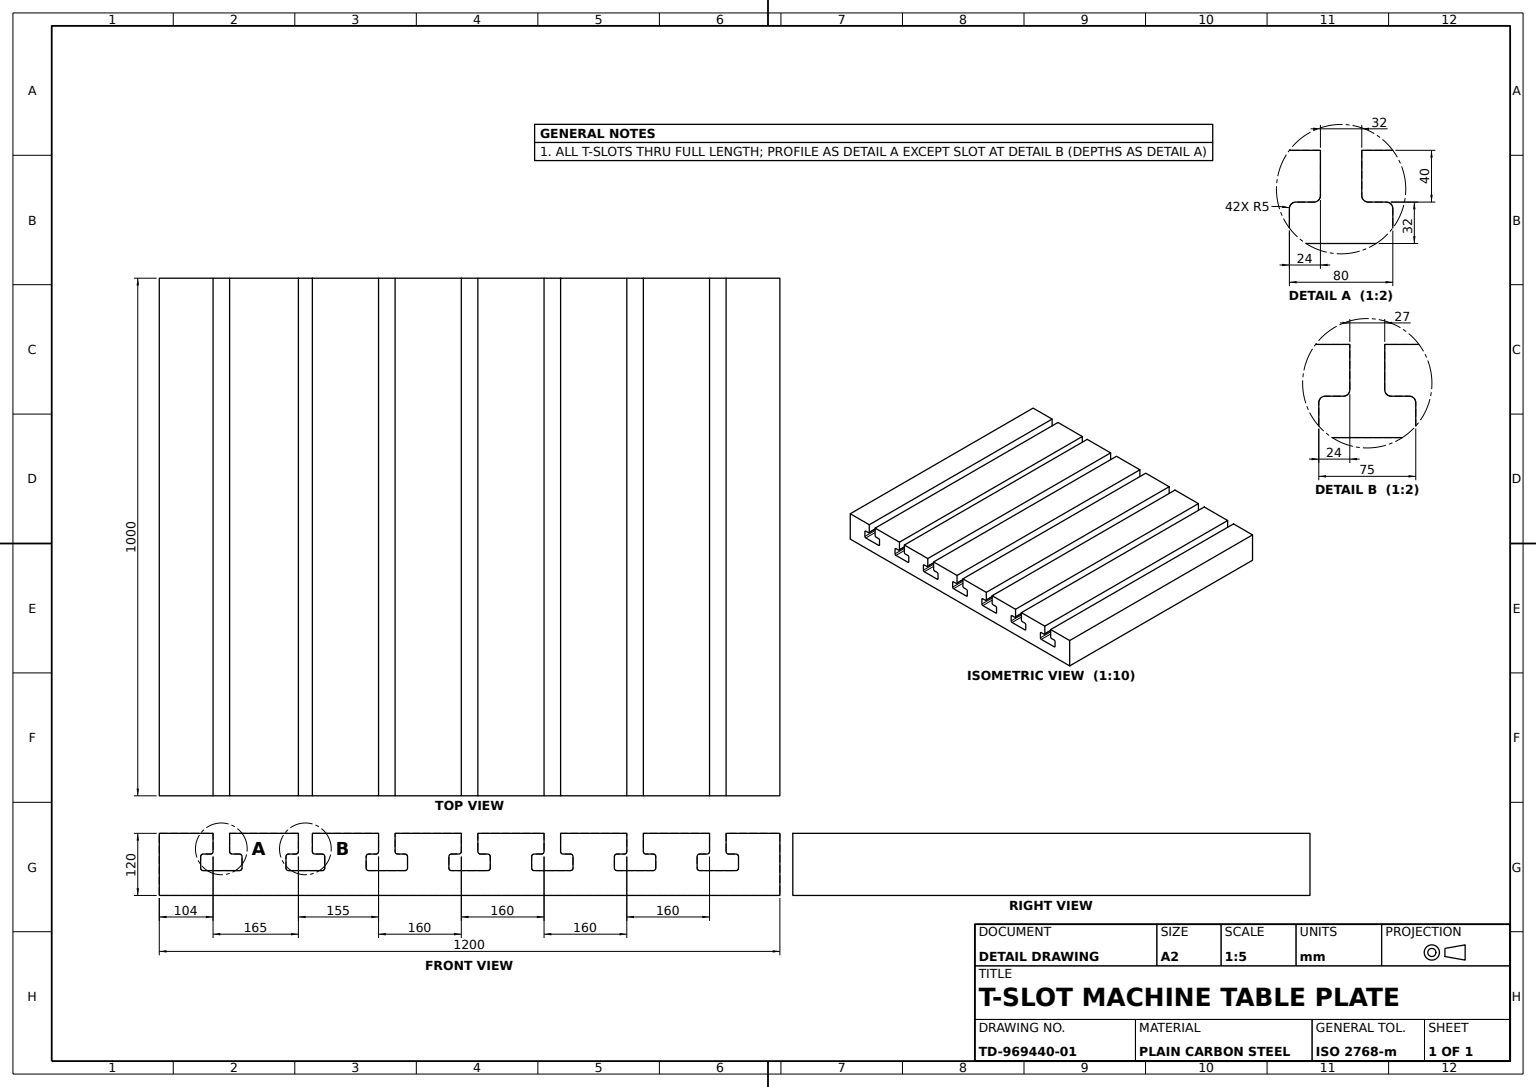
from build123d import *

# Parameters (mm, degrees)
PLATE_OUTLINE_SKETCH_W = 1200
PLATE_OUTLINE_SKETCH_H = 1000
BASE_PLATE_120MM_DEPTH = 120
T_SLOTS_SET_A_DEPTH    = 1000
T_SLOTS_SET_B_DEPTH    = 1000


with BuildPart() as part:
    # Plate Outline Sketch → Base Plate 120mm (new body)
    with BuildSketch(Plane.XY):
        with Locations((600, 500)):
            Rectangle(PLATE_OUTLINE_SKETCH_W, PLATE_OUTLINE_SKETCH_H)
    extrude(amount=BASE_PLATE_120MM_DEPTH)

    # T-Slot Profiles Set A Sketch → T-Slots Set A (cut)
    with BuildSketch(Plane.XZ):
        with BuildLine():
            Line((99, 80), (85, 80))
            ThreePointArc((85, 80), (81.464466094, 78.535533906), (80, 75))
            Line((80, 75), (80, 53))
            ThreePointArc((80, 53), (81.464466094, 49.464466094), (85, 48))
            Line((85, 48), (155, 48))
            ThreePointArc((155, 48), (158.535533906, 49.464466094), (160, 53))
            Line((160, 53), (160, 75))
            ThreePointArc((160, 75), (158.535533906, 78.535533906), (155, 80))
            Line((155, 80), (141, 80))
            ThreePointArc((141, 80), (137.464466094, 81.464466094), (136, 85))
            Line((136, 85), (136, 120))
            Line((136, 120), (104, 120))
            Line((104, 120), (104, 85))
            ThreePointArc((104, 85), (102.535533906, 81.464466094), (99, 80))
        make_face()
    extrude(amount=-T_SLOTS_SET_A_DEPTH, mode=Mode.SUBTRACT)

    # T-Slot Profiles Set B Sketch → T-Slots Set B (cut)
    with BuildSketch(Plane.XZ):
        with BuildLine():
            Line((269, 120), (296, 120))
            Line((296, 120), (296, 85))
            ThreePointArc((296, 85), (297.464466094, 81.464466094), (301, 80))
            Line((301, 80), (315, 80))
            ThreePointArc((315, 80), (318.535533906, 78.535533906), (320, 75))
            Line((320, 75), (320, 53))
            ThreePointArc((320, 53), (318.535533906, 49.464466094), (315, 48))
            Line((315, 48), (280, 48))
            Line((280, 48), (250, 48))
            ThreePointArc((250, 48), (246.464466094, 49.464466094), (245, 53))
            Line((245, 53), (245, 75))
            ThreePointArc((245, 75), (246.464466094, 78.535533906), (250, 80))
            Line((250, 80), (264, 80))
            ThreePointArc((264, 80), (267.535533906, 81.464466094), (269, 85))
            Line((269, 85), (269, 120))
        make_face()
        with BuildLine():
            Line((424, 120), (456, 120))
            Line((456, 120), (456, 85))
            ThreePointArc((456, 85), (457.464466094, 81.464466094), (461, 80))
            Line((461, 80), (475, 80))
            ThreePointArc((475, 80), (478.535533906, 78.535533906), (480, 75))
            Line((480, 75), (480, 53))
            ThreePointArc((480, 53), (478.535533906, 49.464466094), (475, 48))
            Line((475, 48), (440, 48))
            Line((440, 48), (405, 48))
            ThreePointArc((405, 48), (401.464466094, 49.464466094), (400, 53))
            Line((400, 53), (400, 75))
            ThreePointArc((400, 75), (401.464466094, 78.535533906), (405, 80))
            Line((405, 80), (419, 80))
            ThreePointArc((419, 80), (422.535533906, 81.464466094), (424, 85))
            Line((424, 85), (424, 120))
        make_face()
        with BuildLine():
            Line((584, 120), (616, 120))
            Line((616, 120), (616, 85))
            ThreePointArc((616, 85), (617.464466094, 81.464466094), (621, 80))
            Line((621, 80), (635, 80))
            ThreePointArc((635, 80), (638.535533906, 78.535533906), (640, 75))
            Line((640, 75), (640, 53))
            ThreePointArc((640, 53), (638.535533906, 49.464466094), (635, 48))
            Line((635, 48), (600, 48))
            Line((600, 48), (565, 48))
            ThreePointArc((565, 48), (561.464466094, 49.464466094), (560, 53))
            Line((560, 53), (560, 75))
            ThreePointArc((560, 75), (561.464466094, 78.535533906), (565, 80))
            Line((565, 80), (579, 80))
            ThreePointArc((579, 80), (582.535533906, 81.464466094), (584, 85))
            Line((584, 85), (584, 120))
        make_face()
        with BuildLine():
            Line((744, 120), (776, 120))
            Line((776, 120), (776, 85))
            ThreePointArc((776, 85), (777.464466094, 81.464466094), (781, 80))
            Line((781, 80), (795, 80))
            ThreePointArc((795, 80), (798.535533906, 78.535533906), (800, 75))
            Line((800, 75), (800, 53))
            ThreePointArc((800, 53), (798.535533906, 49.464466094), (795, 48))
            Line((795, 48), (760, 48))
            Line((760, 48), (725, 48))
            ThreePointArc((725, 48), (721.464466094, 49.464466094), (720, 53))
            Line((720, 53), (720, 75))
            ThreePointArc((720, 75), (721.464466094, 78.535533906), (725, 80))
            Line((725, 80), (739, 80))
            ThreePointArc((739, 80), (742.535533906, 81.464466094), (744, 85))
            Line((744, 85), (744, 120))
        make_face()
        with BuildLine():
            Line((904, 120), (936, 120))
            Line((936, 120), (936, 85))
            ThreePointArc((936, 85), (937.464466094, 81.464466094), (941, 80))
            Line((941, 80), (955, 80))
            ThreePointArc((955, 80), (958.535533906, 78.535533906), (960, 75))
            Line((960, 75), (960, 53))
            ThreePointArc((960, 53), (958.535533906, 49.464466094), (955, 48))
            Line((955, 48), (920, 48))
            Line((920, 48), (885, 48))
            ThreePointArc((885, 48), (881.464466094, 49.464466094), (880, 53))
            Line((880, 53), (880, 75))
            ThreePointArc((880, 75), (881.464466094, 78.535533906), (885, 80))
            Line((885, 80), (899, 80))
            ThreePointArc((899, 80), (902.535533906, 81.464466094), (904, 85))
            Line((904, 85), (904, 120))
        make_face()
        with BuildLine():
            Line((1064, 120), (1096, 120))
            Line((1096, 120), (1096, 85))
            ThreePointArc((1096, 85), (1097.464466094, 81.464466094), (1101, 80))
            Line((1101, 80), (1115, 80))
            ThreePointArc((1115, 80), (1118.535533906, 78.535533906), (1120, 75))
            Line((1120, 75), (1120, 53))
            ThreePointArc((1120, 53), (1118.535533906, 49.464466094), (1115, 48))
            Line((1115, 48), (1080, 48))
            Line((1080, 48), (1045, 48))
            ThreePointArc((1045, 48), (1041.464466094, 49.464466094), (1040, 53))
            Line((1040, 53), (1040, 75))
            ThreePointArc((1040, 75), (1041.464466094, 78.535533906), (1045, 80))
            Line((1045, 80), (1059, 80))
            ThreePointArc((1059, 80), (1062.535533906, 81.464466094), (1064, 85))
            Line((1064, 85), (1064, 120))
        make_face()
    extrude(amount=-T_SLOTS_SET_B_DEPTH, mode=Mode.SUBTRACT)


solid = part.part
